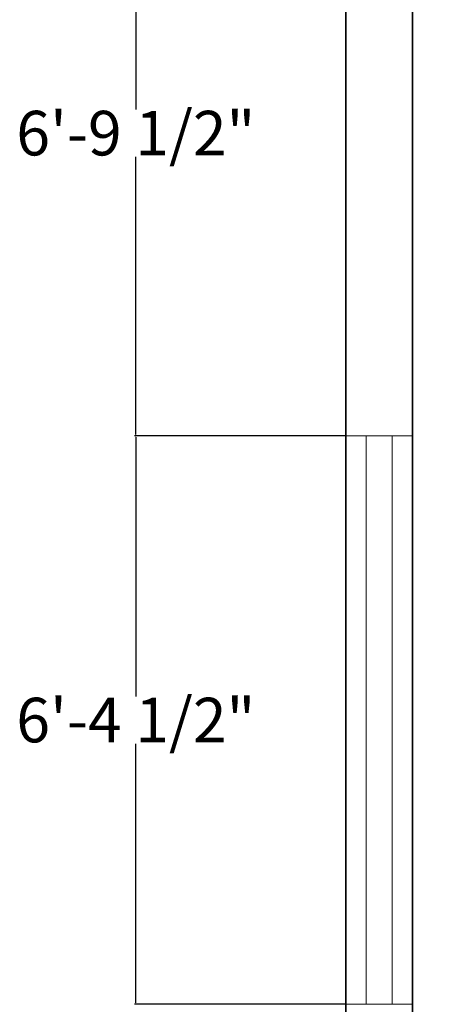
# Model space of a CAD drawing. Units: inches. Extents: x -26 to 575, y -18 to 513.
# Tile 4 of 28: x -26 to 31, y 191 to 324. Entities that reach past the tile are written whole.
import ezdxf

# ---------------------------------------------------------------- set-up
doc = ezdxf.new("R2010")
doc.units = ezdxf.units.IN
doc.header["$MEASUREMENT"] = 0
for name, color, linetype, lineweight in [('A-ANNO-DIMS', 2, 'Continuous', 18), ('A-GLAZ', 4, 'Continuous', 18), ('A-WALL', 7, 'Continuous', 35)]:
    doc.layers.add(name, color=color, linetype=linetype, lineweight=lineweight)
doc.styles.get("Standard").update_dxf_attribs({"font": 'arial.ttf', "height": 6})
doc.dimstyles.get("Standard").update_dxf_attribs({"dimtxt": 6, "dimasz": 0.18, "dimexe": 0.18, "dimexo": 0.0625, "dimgap": 0.09, "dimtad": 0, "dimtih": 1, "dimtoh": 1, "dimzin": 0, "dimdsep": 46, "dimlunit": 3, "dimtxsty": 'Standard', "dimcen": 0.09, "dimadec": 0, "dimazin": 0, "dimtfac": 1, "dimtofl": 0, "dimtmove": 0, "dimatfit": 3, "dimfxl": 1, "dimtolj": 1, "dimtzin": 0, "dimarcsym": 0})

# ---------------------------------------------------------------- blocks, each defined once
blk = doc.blocks.new('*D36')
at = {"layer": 'A-ANNO-DIMS', "color": 0, "lineweight": -2, "transparency": 16777216}
for p, q in [((18.11, 267.49), (-10.3, 267.49)), ((-10.12, 267.31), (-10.12, 232.43)), ((-10.12, 191.16), (-10.12, 226.04)), ((18.11, 190.98), (-10.3, 190.98))]:
    blk.add_line(p, q, dxfattribs=at)
at = {"layer": 'A-ANNO-DIMS', "color": 0, "transparency": 16777216}
for points in [[(-10.15, 267.31), (-10.09, 267.31), (-10.12, 267.49)], [(-10.15, 191.16), (-10.09, 191.16), (-10.12, 190.98)]]:
    blk.add_solid(points, dxfattribs=at)
at = {"layer": 'Defpoints', "color": 0, "transparency": 16777216}
for p in [(-10.12, 267.49), (18.18, 267.49), (18.18, 190.98)]:
    blk.add_point(p, dxfattribs=at)
at = {"layer": 'A-ANNO-DIMS', "color": 0, "transparency": 16777216, "insert": (-10.12, 229.24), "char_height": 6, "attachment_point": 5}
blk.add_mtext('\\A1;6\'-4 1/2"', dxfattribs=at)
blk = doc.blocks.new('*D37')
at = {"layer": 'A-ANNO-DIMS', "color": 0, "lineweight": -2, "transparency": 16777216}
for p, q in [((18.11, 348.99), (-10.3, 348.99)), ((-10.12, 348.81), (-10.12, 311.43)), ((-10.12, 267.67), (-10.12, 305.05)), ((18.11, 267.49), (-10.3, 267.49))]:
    blk.add_line(p, q, dxfattribs=at)
at = {"layer": 'A-ANNO-DIMS', "color": 0, "transparency": 16777216}
for points in [[(-10.15, 348.81), (-10.09, 348.81), (-10.12, 348.99)], [(-10.15, 267.67), (-10.09, 267.67), (-10.12, 267.49)]]:
    blk.add_solid(points, dxfattribs=at)
at = {"layer": 'Defpoints', "color": 0, "transparency": 16777216}
for p in [(-10.12, 348.99), (18.18, 348.99), (18.18, 267.49)]:
    blk.add_point(p, dxfattribs=at)
at = {"layer": 'A-ANNO-DIMS', "color": 0, "transparency": 16777216, "insert": (-10.12, 308.24), "char_height": 6, "attachment_point": 5}
blk.add_mtext('\\A1;6\'-9 1/2"', dxfattribs=at)
blk = doc.blocks.new('*D50')
at = {"layer": 'A-ANNO-DIMS', "color": 0, "lineweight": -2, "transparency": 16777216}
for p, q in [((27.18, 466.45), (27.18, -8.97)), ((58.22, 466.45), (58.22, -8.97)), ((27.36, -8.79), (34.58, -8.79)), ((58.04, -8.79), (50.82, -8.79))]:
    blk.add_line(p, q, dxfattribs=at)
at = {"layer": 'A-ANNO-DIMS', "color": 0, "transparency": 16777216}
for points in [[(27.36, -8.76), (27.36, -8.82), (27.18, -8.79)], [(58.04, -8.76), (58.04, -8.82), (58.22, -8.79)]]:
    blk.add_solid(points, dxfattribs=at)
at = {"layer": 'Defpoints', "color": 0, "transparency": 16777216}
for p in [(27.18, 466.51), (58.22, 466.51), (58.22, -8.79)]:
    blk.add_point(p, dxfattribs=at)
at = {"layer": 'A-ANNO-DIMS', "color": 0, "transparency": 16777216, "insert": (42.7, -8.79), "char_height": 6, "attachment_point": 5}
blk.add_mtext('\\A1;2\'-7"', dxfattribs=at)

msp = doc.modelspace()

# ---------------------------------------------------------------- linework, layer by layer
at = {"layer": 'A-GLAZ'}
for p, q in [((27.177, 267.494), (18.177, 267.494)), ((18.177, 267.494), (18.177, 190.977)), ((20.927, 267.494), (20.927, 190.977)), ((27.177, 267.494), (22.677, 267.494)), ((24.427, 267.494), (24.427, 190.977)), ((27.177, 190.977), (27.177, 267.494)), ((18.177, 190.977), (27.177, 190.977))]:
    msp.add_line(p, q, dxfattribs=at)
at = {"layer": 'A-WALL'}
msp.add_line((27.177, 330.008), (27.177, 127.508), dxfattribs=at)
msp.add_lwpolyline([(18.177, 19.508), (522.177, 19.508), (522.177, 475.508), (18.177, 475.508)], close=True, dxfattribs=at)

# ---------------------------------------------------------------- dimensions: what is measured, and where the dimension line sits
at = {"layer": 'A-ANNO-DIMS'}
dim = msp.add_linear_dim(base=(58.224, -8.792), p1=(27.177, 466.508), p2=(58.224, 466.508), dimstyle='Standard', override={"dimdec": 1, "dimlfac": 1, "dimrnd": 0, "dimzin": 1, "dimdsep": 46, "dimlunit": 4, "dimfrac": 2}, dxfattribs=at)
dim.commit()
dim.dimension.update_dxf_attribs({"geometry": '*D50', "text_midpoint": (42.7, -8.792)})
for base, p1, p2, picture, middle in [((-10.123, 348.988), (18.177, 267.494), (18.177, 348.988), '*D37', (-10.123, 308.241)), ((-10.123, 267.494), (18.177, 190.977), (18.177, 267.494), '*D36', (-10.123, 229.236))]:
    dim = msp.add_linear_dim(base=base, p1=p1, p2=p2, angle=90, dimstyle='Standard', override={"dimdec": 1, "dimlfac": 1, "dimrnd": 0, "dimzin": 1, "dimdsep": 46, "dimlunit": 4, "dimfrac": 2}, dxfattribs=at)
    dim.commit()
    dim.dimension.update_dxf_attribs({"geometry": picture, "text_midpoint": middle})

doc.saveas('drawing.dxf')
